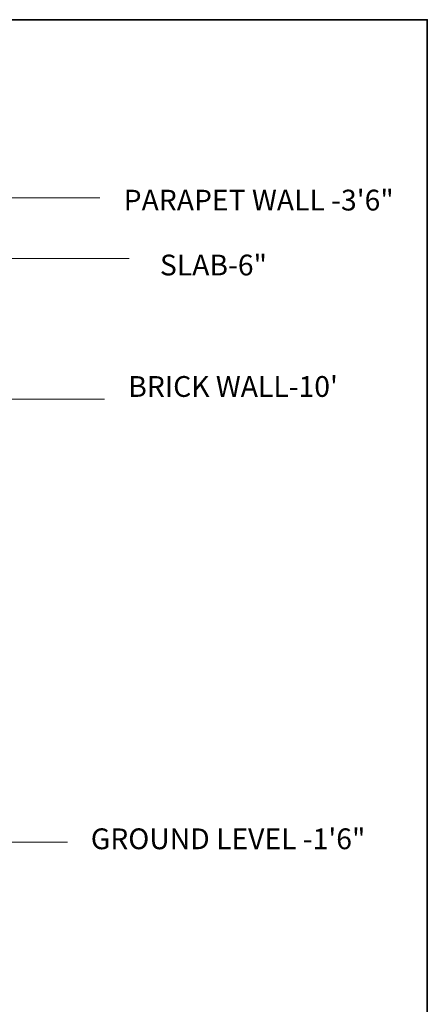
# Model space of a CAD drawing. Units: inches. Extents: x 2416 to 3391, y 1375 to 2496.
# Tile 13 of 13: x 3215 to 3391, y 2069 to 2496. Entities that reach past the tile are written whole.
import ezdxf

# ---------------------------------------------------------------- set-up
doc = ezdxf.new("R2010")
doc.units = ezdxf.units.IN
doc.layers.add('A-ANNO-TEXT', color=7, linetype='Continuous', lineweight=18)
doc.layers.add('A-ANNO-TTLB', color=7, linetype='Continuous', lineweight=35)
doc.styles.get("Standard").update_dxf_attribs({"font": 'arial.ttf'})

msp = doc.modelspace()

# ---------------------------------------------------------------- linework, layer by layer
at = {"layer": 'A-ANNO-TEXT'}
for p, q in [((3202.6924, 2418.8281), (3249.1878, 2418.8281)), ((3199.1027, 2392.591), (3262.0173, 2392.591)), ((3202.6924, 2331.6911), (3251.2079, 2331.6911)), ((3195.1943, 2139.7132), (3235.2126, 2139.7132))]:
    msp.add_line(p, q, dxfattribs=at)
at = {"layer": 'A-ANNO-TTLB'}
msp.add_lwpolyline([(2416.4678, 2496.0939), (3391.2022, 2496.0939), (3391.2022, 1375.1104), (2416.4678, 1375.1104)], close=True, dxfattribs=at)

# ---------------------------------------------------------------- texts
at = {"layer": 'A-ANNO-TEXT', "char_height": 9, "attachment_point": 1}
for s, width, insert in [('PARAPET WALL -3\'6"', 226.258856, (3259.5856, 2422.4071)), ('SLAB-6"', 71.182539, (3275.2937, 2394.2783)), ("BRICK WALL-10'", 97.768775, (3261.5717, 2341.6421)), ('GROUND LEVEL -1\'6"', 164.494285, (3245.3309, 2145.6229))]:
    msp.add_mtext_dynamic_manual_height_columns(s, width=width, gutter_width=12.5, heights=[0], dxfattribs=dict(at, insert=insert))

doc.saveas('drawing.dxf')
